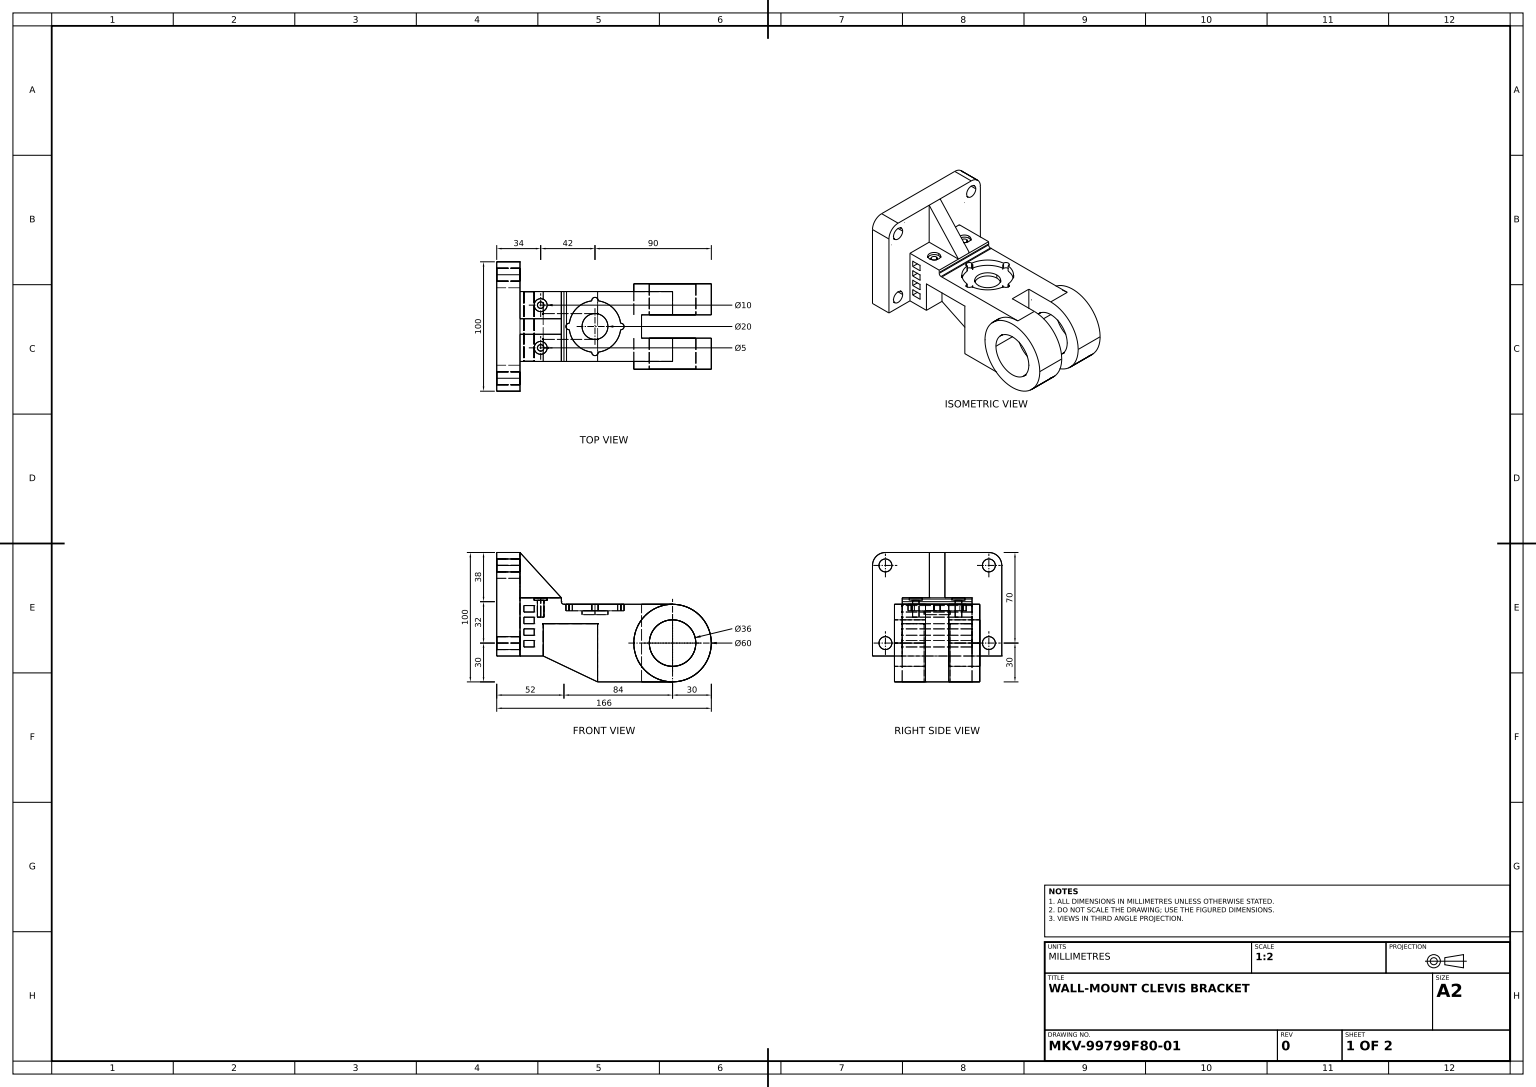
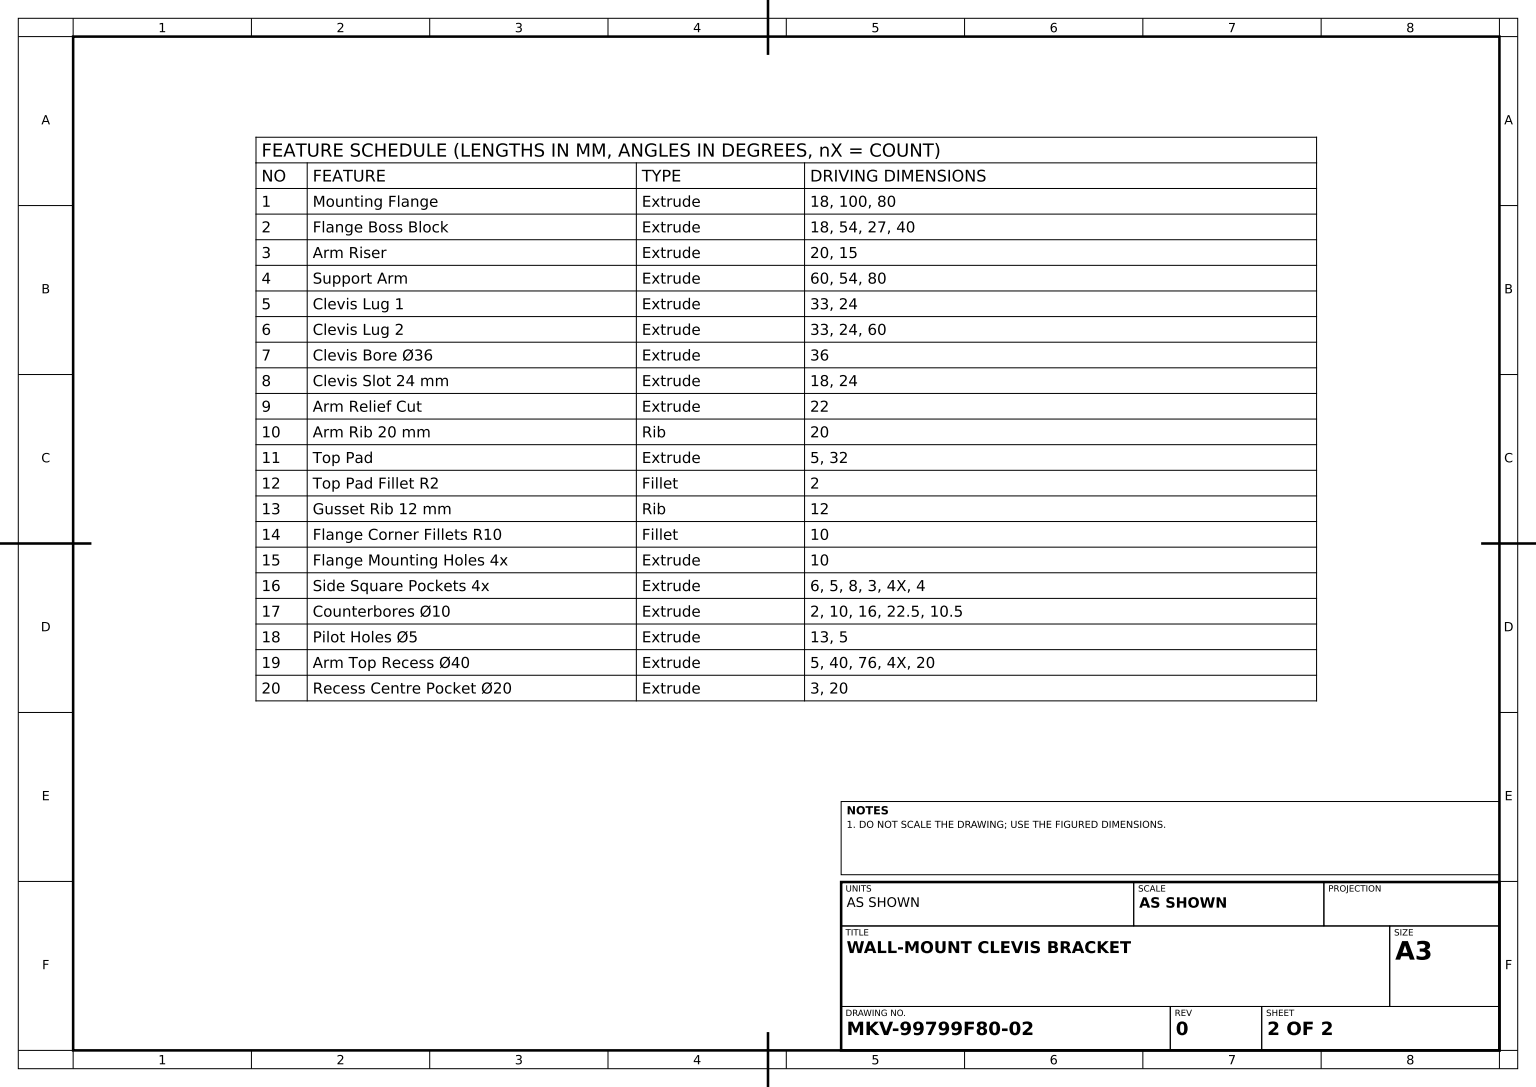
SolidWorks part; units mm, degrees
material "Plain Carbon Steel"
ref_plane "Front Plane" through (0, 0, 0) normal (0, 0, 1) x (1, 0, 0)
ref_plane "Top Plane" through (0, 0, 0) normal (0, 1, 0) x (1, 0, 0)
ref_plane "Right Plane" through (0, 0, 0) normal (1, 0, 0) x (0, 0, -1)
sketch "Mounting Flange Sketch" plane through (0, 0, 0) normal (1, 0, 0) x (0, 0, -1)
  line L1 (-50, -40) -> (50, -40)
  line L2 (-50, -40) -> (-50, 40)
  line L3 (-50, 40) -> (50, 40)
  line L4 (50, -40) -> (50, 40)
  line L5 (-50, -40) -> (50, 40) construction
  line L6 (-50, 40) -> (50, -40) construction
  point P0 (0, 0)
  dimension "D1" = 100
  dimension "D2" = 80
extrude "Mounting Flange" add sketch "Mounting Flange Sketch" along normal blind 18
sketch "Flange Boss Block Sketch" plane through (18, 0, 0) normal (1, 0, 0) x (0, 0, -1)
  line L0 (-50, -40) -> (50, -40) construction
  line L1 (-27, -40) -> (27, -40)
  line L2 (-27, -40) -> (-27, 0)
  line L3 (-27, 0) -> (27, 0)
  line L4 (27, -40) -> (27, 0)
  dimension "D1" = 54
  dimension "D2" = 27
  dimension "D3" = 40
extrude "Flange Boss Block" add sketch "Flange Boss Block Sketch" along normal blind 18
sketch "Arm Riser Sketch" plane through (36, 0, 0) normal (1, 0, 0) x (0, 0, -1)
  line L0 (27, -40) -> (27, 0) construction
  line L1 (-27, 0) -> (27, 0)
  line L2 (-27, 0) -> (-27, -15)
  line L3 (-27, -15) -> (27, -15)
  line L4 (27, 0) -> (27, -15)
  dimension "D1" = 15
extrude "Arm Riser" add sketch "Arm Riser Sketch" along normal blind 20
sketch "Support Arm Sketch" plane through (0, 0, 0) normal (0, 1, 0) x (1, 0, 0)
  line L1 (56, 27) -> (136, 27)
  line L2 (56, 27) -> (56, -27)
  line L3 (56, -27) -> (136, -27)
  line L4 (136, 27) -> (136, -27)
  dimension "D1" = 54
  dimension "D2" = 80
extrude "Support Arm" add sketch "Support Arm Sketch" against normal blind 60
ref_plane "Plane1" through (0, 0, 33) normal (0, 0, 1) x (1, 0, 0)
sketch "Clevis Lug 1 Sketch" plane through (0, 0, 33) normal (0, 0, 1) x (1, 0, 0)
  line L0 (136, -60) -> (136, 0) construction
  circle A0 centre (136, -30) radius 30
extrude "Clevis Lug 1" add sketch "Clevis Lug 1 Sketch" against normal blind 24
ref_plane "Plane2" through (0, 0, -33) normal (0, 0, 1) x (1, 0, 0)
sketch "Clevis Lug 2 Sketch" plane through (0, 0, -33) normal (0, 0, 1) x (1, 0, 0)
  line L0 (136, 0) -> (136, -60) construction
  circle A0 centre (136, -30) radius 30
  dimension "D1" = 60
extrude "Clevis Lug 2" add sketch "Clevis Lug 2 Sketch" along normal blind 24
sketch "Clevis Bore Sketch" plane through (0, 0, 33) normal (0, 0, 1) x (1, 0, 0)
  circle A0 centre (136, -30) radius 18
  dimension "D1" = 36
extrude "Clevis Bore Ø36" cut sketch "Clevis Bore Sketch" against normal through all
sketch "Clevis Slot Sketch" plane through (0, 0, 0) normal (0, 1, 0) x (1, 0, 0)
  line L1 (136, 9) -> (112, 9)
  line L2 (136, 9) -> (136, -9)
  line L3 (136, -9) -> (112, -9)
  line L4 (112, 9) -> (112, -9)
  dimension "D1" = 18
  dimension "D2" = 24
extrude "Clevis Slot 24 mm" cut sketch "Clevis Slot Sketch" against normal through all
sketch "Arm Relief Cut Sketch" plane through (0, 0, 27) normal (0, 0, 1) x (1, 0, 0)
  line L0 (56, -60) -> (136, -60) construction
  line L1 (56, -15) -> (78, -15)
  line L2 (56, -15) -> (56, -60)
  line L3 (56, -60) -> (78, -60)
  line L4 (78, -15) -> (78, -60)
  dimension "D1" = 22
extrude "Arm Relief Cut" cut sketch "Arm Relief Cut Sketch" against normal through all
ref_plane "Plane3" through (0, 0, 0) normal (0, 0, 1) x (1, 0, 0)
sketch "Arm Rib Sketch" plane through (0, 0, 0) normal (0, 0, 1) x (1, 0, 0)
  line L0 (36, -40) -> (78, -60)
rib "Arm Rib 20 mm" sketch "Arm Rib Sketch" sketch "Arm Rib Sketch" thickness 20 extrusion direction parallel to sketch draft on no parameters "D1"=20
sketch "Top Pad Sketch" plane through (0, 0, 0) normal (0, 1, 0) x (1, 0, 0)
  line L0 (136, -27) -> (18, -27) construction
  line L1 (18, 27) -> (50, 27)
  line L2 (18, 27) -> (18, -27)
  line L3 (18, -27) -> (50, -27)
  line L4 (50, 27) -> (50, -27)
  dimension "D1" = 32
extrude "Top Pad" add sketch "Top Pad Sketch" along normal blind 5
fillet "Top Pad Fillet R2" radius 2 1 edges at (50, 0, 0)
ref_plane "Plane5" through (0, 0, 0) normal (0, 0, 1) x (1, 0, 0)
sketch "Gusset Rib Sketch" plane through (0, 0, 0) normal (0, 0, 1) x (1, 0, 0)
  line L0 (18, 40) -> (50, 5)
rib "Gusset Rib 12 mm" sketch "Gusset Rib Sketch" sketch "Gusset Rib Sketch" thickness 12 extrusion direction parallel to sketch draft on no parameters "D1"=12
fillet "Flange Corner Fillets R10" radius 10 2 edges at (9, 40, -50) (9, 40, 50)
sketch "Flange Mounting Holes Sketch" plane through (18, 0, 0) normal (1, 0, 0) x (0, 0, -1)
  line L0 (-50, -40) -> (-27, -40) construction
  line L1 (-50, 30) -> (-50, -40) construction
  line L2 (50, -40) -> (50, 30) construction
  line L3 (27, -40) -> (50, -40) construction
  circle A0 centre (-40, 30) radius 5
  circle A1 centre (40, 30) radius 5
  circle A2 centre (-40, -30) radius 5
  circle A3 centre (40, -30) radius 5
  dimension "D1" = 10
  dimension "D2" = 10
  dimension "D3" = 10
  dimension "D4" = 10
  dimension "D5" = 10
  dimension "D6" = 10
  dimension "D7" = 10
  dimension "D8" = 10
extrude "Flange Mounting Holes 4x" cut sketch "Flange Mounting Holes Sketch" against normal through all
sketch "Side Square Pockets Sketch" plane through (0, 0, 27) normal (0, 0, 1) x (1, 0, 0)
  line L0 (18, 5) -> (50, 5) construction
  line L1 (21, -1) -> (29, -1)
  line L2 (21, -1) -> (21, -6)
  line L3 (21, -6) -> (29, -6)
  line L4 (29, -1) -> (29, -6)
  line L5 (18, 30) -> (18, -40) construction
  line L6 (21, -15) -> (29, -15)
  line L7 (29, -10) -> (29, -15)
  line L8 (21, -10) -> (29, -10)
  line L9 (21, -10) -> (21, -15)
  line L10 (21, -24) -> (29, -24)
  line L11 (29, -19) -> (29, -24)
  line L12 (21, -19) -> (29, -19)
  line L13 (21, -19) -> (21, -24)
  line L14 (21, -33) -> (29, -33)
  line L15 (29, -28) -> (29, -33)
  line L16 (21, -28) -> (29, -28)
  line L17 (21, -28) -> (21, -33)
  dimension "D1" = 6
  dimension "D2" = 5
  dimension "D3" = 8
  dimension "D4" = 3
  dimension "D6" = 4
  dimension "D5" = 4
extrude "Side Square Pockets 4x" cut sketch "Side Square Pockets Sketch" against normal through all and the other way through all
sketch "Counterbore Sketch" plane through (0, 5, 0) normal (0, 1, 0) x (1, 0, 0)
  line L0 (18, -6) -> (18, -27) construction
  line L1 (18, -6) -> (50, -6) construction
  circle A0 centre (34, -16.5) radius 5
  circle A1 centre (34, 16.5) radius 5
  dimension "D1" = 10
  dimension "D2" = 10
  dimension "D3" = 16
  dimension "D4" = 22.5
  dimension "D5" = 10.5
extrude "Counterbores Ø10" cut sketch "Counterbore Sketch" against normal blind 2
sketch "Pilot Holes Sketch" plane through (0, 3, 0) normal (0, 1, 0) x (1, 0, 0)
  circle A0 centre (34, 16.5) radius 2.5
  circle A1 centre (34, -16.5) radius 2.5
  dimension "D1" = 5
  dimension "D2" = 5
extrude "Pilot Holes Ø5" cut sketch "Pilot Holes Sketch" against normal blind 13
sketch "Arm Top Recess Sketch" plane through (0, 0, 0) normal (0, 1, 0) x (1, 0, 0)
  arc A0 (73.5049, 19.8438) -> (56.1562, 2.4951) centre (76, 0) ccw
  arc A1 (56.1562, 2.4951) -> (56.1562, -2.4951) centre (56, 0) ccw
  arc A2 (78.4951, 19.8438) -> (73.5049, 19.8438) centre (76, 20) ccw
  arc A3 (95.8437, -2.4951) -> (95.8438, 2.4951) centre (96, 0) ccw
  arc A4 (73.5049, -19.8437) -> (78.4951, -19.8437) centre (76, -20) ccw
  arc A5 (56.1562, -2.4951) -> (73.5049, -19.8437) centre (76, 0) ccw
  arc A6 (78.4951, -19.8437) -> (95.8437, -2.4951) centre (76, 0) ccw
  arc A7 (95.8438, 2.4951) -> (78.4951, 19.8438) centre (76, 0) ccw
  dimension "D1" = 40
  dimension "D3" = 5
  dimension "D6" = 20
  dimension "D2" = 76
  dimension "D5" = 40
  dimension "D7" = 20
  dimension "D4" = 4
extrude "Arm Top Recess Ø40" cut sketch "Arm Top Recess Sketch" against normal blind 5
sketch "Recess Centre Pocket Sketch" plane through (0, -5, 0) normal (0, 1, 0) x (1, 0, 0)
  circle A0 centre (76, 0) radius 10
  dimension "D1" = 20
extrude "Recess Centre Pocket Ø20" cut sketch "Recess Centre Pocket Sketch" against normal blind 3
